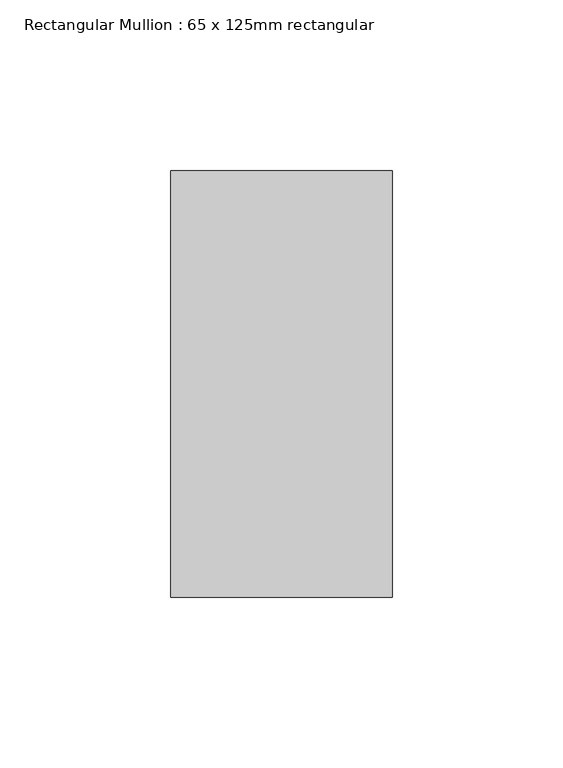
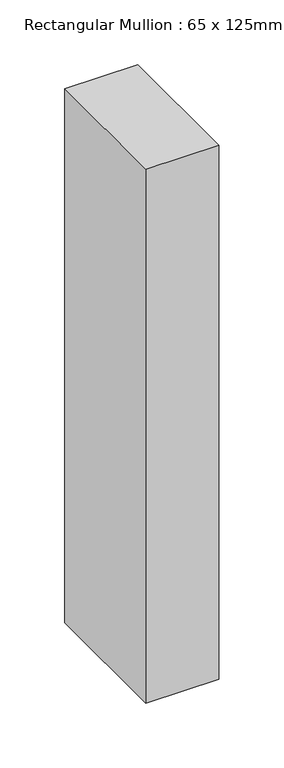
"""IFC4 building model written with IfcOpenShell, lengths in millimetres: member geometry, Rectangular Mullion : 65 x 125mm rectangular."""

from ifc_helpers import new_model, si_unit, frame, origin, place, context, project, spatial, polyline, outline, extrude, source, transform, mapped, element, save


def rectangular_mullion_65_x_125mm_rectangular_623ff0e3(model_context):
    return source(origin(), model_context, "Body", "SweptSolid", [
        extrude(outline(polyline([(0.0, 62.5), (0.0, -62.5), (-65.0, -62.5), (-65.0, 62.5), (0.0, 62.5)])), frame((0.0, 0.0, -502.5), z_axis=(0.0, 0.0, 1.0), x_axis=(1.0, 0.0, 0.0)), (0.0, 0.0, 1.0), 502.5),
    ])


if __name__ == "__main__":
    model = new_model("IFC4")
    model_context = context("Model", 3, world=origin())
    ifc_project = project(units=[si_unit("LENGTHUNIT", "METRE", prefix="MILLI")], contexts=[model_context])
    site = spatial("IfcSite", under=ifc_project)
    building = spatial("IfcBuilding", under=site)
    placement = place(None, origin())
    rectangular_mullion_65_x_125mm_rectangular_shape = rectangular_mullion_65_x_125mm_rectangular_623ff0e3(model_context)
    element("IfcMember", 1, ObjectType="Rectangular Mullion : 65 x 125mm rectangular", at=placement, inside=building, context=model_context, shape_type="MappedRepresentation", body=[
        mapped(rectangular_mullion_65_x_125mm_rectangular_shape, transform((0.0, 0.0, 0.0), x_axis=(1.0, 0.0, 0.0), y_axis=(0.0, 1.0, 0.0), z_axis=(0.0, 0.0, 1.0))),
    ])
    save(model, "model.ifc")

# Revit data of these elements
# Type "Rectangular Mullion : 65 x 125mm rectangular"
#   built-in parameter 1007304 = 0.410105 (stored number, unit not read)
#   built-in parameter 1007301 = 0.106627 (stored number, unit not read)
#   built-in parameter 1007300 = 0.106627 (stored number, unit not read)
# Element 1 (IfcMember, "Rectangular Mullion : 65 x 125mm rectangular")
#   Materials on its faces: "Aluminum"
# Materials
#   "Aluminum": class "Metal", colour RGB 244 245 246, transparency 0, Description = "Aluminum 6061", Cost = 0
